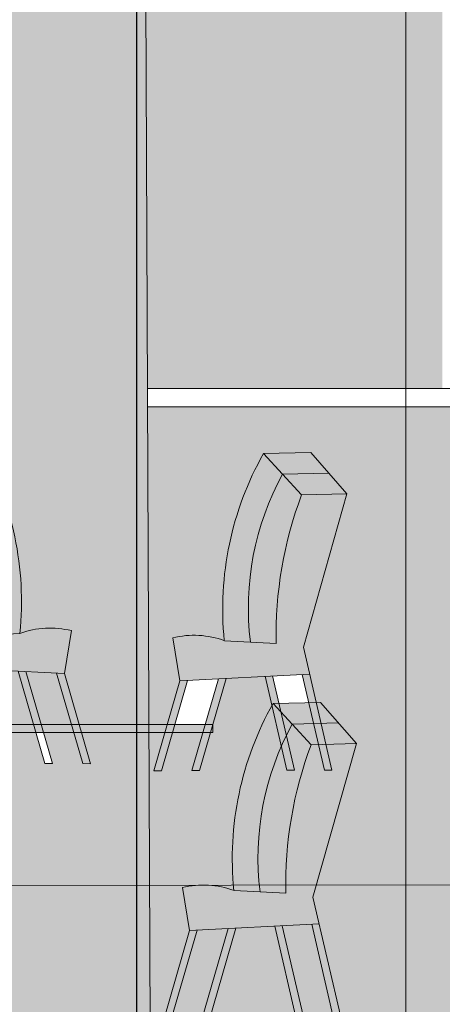
# Model space of a CAD drawing. Units: millimetres. Extents: x 11032 to 26788, y 3406 to 24505.
# Tile 10 of 78: x 16566 to 17145, y 7421 to 8770. Entities that reach past the tile are written whole.
import ezdxf

# ---------------------------------------------------------------- set-up
doc = ezdxf.new("R2010")
doc.units = ezdxf.units.MM
doc.header["$MEASUREMENT"] = 0
for name, color, linetype, lineweight in [('A-ANNO-DIMS', 2, 'Continuous', 18), ('A-FURN', 8, 'Continuous', 13), ('A-FURN-PATT', 8, 'Continuous', 13), ('A-GLAZ', 250, 'Continuous', 20), ('A-WALL-INTR', 8, 'Continuous', 18)]:
    doc.layers.add(name, color=color, linetype=linetype, lineweight=lineweight)
doc.layers.add('A-GLAZ-FRAM-PATT', color=250, linetype='Continuous', lineweight=13, true_color=0x262627)
doc.layers.add('A-WALL-INTR-PATT', color=251, linetype='Continuous', lineweight=13, true_color=0x6c6b6a)
doc.styles.get("Standard").update_dxf_attribs({"font": 'arial.ttf'})
doc.dimstyles.get("Standard").update_dxf_attribs({"dimtxt": 150, "dimasz": 100, "dimexe": 10, "dimexo": 5, "dimgap": 5, "dimtad": 0, "dimtih": 1, "dimtoh": 1, "dimdec": 0, "dimzin": 0, "dimdsep": 46, "dimtxsty": 'Standard', "dimcen": 0.09, "dimadec": 0, "dimazin": 0, "dimtfac": 1, "dimtdec": 0, "dimtofl": 0, "dimtmove": 0, "dimatfit": 3, "dimfxl": 1, "dimtolj": 1, "dimtzin": 0, "dimarcsym": 0})

# ---------------------------------------------------------------- blocks, each defined once
blk = doc.blocks.new('DINING-CHAIR-ELEV')
blk.add_line((228.7, 123.4), (51, 132.6))
for points in [[(0, 379.5), (49.4, 435.9), (114.1, 434.5)], [(61.2, 132.1), (30.8, 1.2), (20.5, 1.2), (59.5, 169.3), (0, 379.5), (61.9, 377.9)], [(111.9, 129.5), (82.1, 0.9), (71.8, 1), (101.8, 130)], [(165.3, 126.7), (201.8, 0.3), (212.2, 0.3), (175.8, 126.2)]]:
    blk.add_lwpolyline(points)
for points in [[(218.1, 124), (253.9, 0.1), (264.3, 0), (228.7, 123.4), (238.3, 182.2, 0.148451), (167.5, 178.3), (96.6, 174.5, 0.097012), (61.9, 377.9), (114.1, 434.5, -0.154833), (167.8, 178.5)], [(132, 176.4, 0.156877), (88, 406.2), (24.7, 407.7)]]:
    blk.add_lwpolyline(points, format="xyb")
blk = doc.blocks.new('DINING-TABLE-ELEV')
blk.add_lwpolyline([(0, 0), (986.1, 0), (986.1, 11.1), (0, 11.1)], close=True)
blk = doc.blocks.new('*D17')
at = {"layer": 'A-ANNO-DIMS', "color": 0, "lineweight": -2, "transparency": 16777216}
for p, q in [((15472.4, 7380.1), (15472.4, 7309.7)), ((15736.7, 7380.1), (15736.7, 7309.7)), ((15572.4, 7319.7), (15636.7, 7319.7)), ((15736.7, 7319.7), (15836.7, 7319.7))]:
    blk.add_line(p, q, dxfattribs=at)
at = {"layer": 'A-ANNO-DIMS', "color": 0, "transparency": 16777216}
for points in [[(15572.4, 7336.4), (15572.4, 7303), (15472.4, 7319.7)], [(15636.7, 7336.4), (15636.7, 7303), (15736.7, 7319.7)]]:
    blk.add_solid(points, dxfattribs=at)
at = {"layer": 'Defpoints', "color": 0, "transparency": 16777216}
for p in [(15472.4, 7385.1), (15736.7, 7385.1), (15736.7, 7319.7)]:
    blk.add_point(p, dxfattribs=at)
at = {"layer": 'A-ANNO-DIMS', "color": 0, "transparency": 16777216, "insert": (16266.4, 7319.7), "char_height": 150, "attachment_point": 5}
blk.add_mtext('\\A1;264 TYP.', dxfattribs=at)
blk = doc.blocks.new('*D36')
at = {"layer": 'A-ANNO-DIMS', "color": 0, "lineweight": -2, "transparency": 16777216}
for p, q in [((12301.3, 17115.9), (12301.3, 24416.9)), ((12401.3, 24406.9), (18569.2, 24406.9)), ((25297.4, 24406.9), (19129.5, 24406.9)), ((25397.4, 4466.4), (25397.4, 24416.9))]:
    blk.add_line(p, q, dxfattribs=at)
at = {"layer": 'A-ANNO-DIMS', "color": 0, "transparency": 16777216}
for points in [[(12401.3, 24423.5), (12401.3, 24390.2), (12301.3, 24406.9)], [(25297.4, 24423.5), (25297.4, 24390.2), (25397.4, 24406.9)]]:
    blk.add_solid(points, dxfattribs=at)
at = {"layer": 'Defpoints', "color": 0, "transparency": 16777216}
for p in [(25397.4, 24406.9), (12301.3, 17110.9), (25397.4, 4461.4)]:
    blk.add_point(p, dxfattribs=at)
at = {"layer": 'A-ANNO-DIMS', "color": 0, "transparency": 16777216, "insert": (18849.3, 24406.9), "char_height": 150, "attachment_point": 5}
blk.add_mtext('\\A1;13096', dxfattribs=at)
blk = doc.blocks.new('*D37')
at = {"layer": 'A-ANNO-DIMS', "color": 0, "lineweight": -2, "transparency": 16777216}
for p, q in [((18087.7, 23450.4), (11334.8, 23450.4)), ((11344.8, 23350.4), (11344.8, 14037.5)), ((11344.8, 4561.4), (11344.8, 13874.3)), ((12927.7, 4461.4), (11334.8, 4461.4))]:
    blk.add_line(p, q, dxfattribs=at)
at = {"layer": 'A-ANNO-DIMS', "color": 0, "transparency": 16777216}
for points in [[(11328.1, 23350.4), (11361.4, 23350.4), (11344.8, 23450.4)], [(11328.1, 4561.4), (11361.4, 4561.4), (11344.8, 4461.4)]]:
    blk.add_solid(points, dxfattribs=at)
at = {"layer": 'Defpoints', "color": 0, "transparency": 16777216}
for p in [(11344.8, 23450.4), (18092.7, 23450.4), (12932.7, 4461.4)]:
    blk.add_point(p, dxfattribs=at)
at = {"layer": 'A-ANNO-DIMS', "color": 0, "transparency": 16777216, "insert": (11344.8, 13955.9), "char_height": 150, "attachment_point": 5}
blk.add_mtext('\\A1;18989', dxfattribs=at)
blk = doc.blocks.new('*D49')
at = {"layer": 'A-ANNO-DIMS', "color": 0, "lineweight": -2, "transparency": 16777216}
for p, q in [((17953.5, 10206.4), (17953.5, 3494.9)), ((14996.4, 6406.4), (14996.4, 3494.9)), ((15096.4, 3504.9), (16244.7, 3504.9)), ((17853.5, 3504.9), (16705.2, 3504.9))]:
    blk.add_line(p, q, dxfattribs=at)
at = {"layer": 'A-ANNO-DIMS', "color": 0, "transparency": 16777216}
for points in [[(15096.4, 3521.6), (15096.4, 3488.2), (14996.4, 3504.9)], [(17853.5, 3521.6), (17853.5, 3488.2), (17953.5, 3504.9)]]:
    blk.add_solid(points, dxfattribs=at)
at = {"layer": 'Defpoints', "color": 0, "transparency": 16777216}
for p in [(17953.5, 10211.4), (14996.4, 6411.4), (17953.5, 3504.9)]:
    blk.add_point(p, dxfattribs=at)
at = {"layer": 'A-ANNO-DIMS', "color": 0, "transparency": 16777216, "insert": (16474.9, 3504.9), "char_height": 150, "attachment_point": 5}
blk.add_mtext('\\A1;2957', dxfattribs=at)
blk = doc.blocks.new('*D57')
at = {"layer": 'A-ANNO-DIMS', "color": 0, "lineweight": -2, "transparency": 16777216}
for p, q in [((14994.7, 7266.4), (14994.7, 24416.9)), ((15094.7, 24406.9), (17716, 24406.9)), ((20794.7, 24406.9), (18173.4, 24406.9)), ((20894.7, 7266.4), (20894.7, 24416.9))]:
    blk.add_line(p, q, dxfattribs=at)
at = {"layer": 'A-ANNO-DIMS', "color": 0, "transparency": 16777216}
for points in [[(15094.7, 24423.5), (15094.7, 24390.2), (14994.7, 24406.9)], [(20794.7, 24423.5), (20794.7, 24390.2), (20894.7, 24406.9)]]:
    blk.add_solid(points, dxfattribs=at)
at = {"layer": 'Defpoints', "color": 0, "transparency": 16777216}
for p in [(20894.7, 24406.9), (14994.7, 7261.4), (20894.7, 7261.4)]:
    blk.add_point(p, dxfattribs=at)
at = {"layer": 'A-ANNO-DIMS', "color": 0, "transparency": 16777216, "insert": (17944.7, 24406.9), "char_height": 150, "attachment_point": 5}
blk.add_mtext('\\A1;5900', dxfattribs=at)
blk = doc.blocks.new('*D66')
at = {"layer": 'A-ANNO-DIMS', "color": 0, "lineweight": -2, "transparency": 16777216}
for p, q in [((16725.9, 10296), (16725.9, 3494.9)), ((19150.9, 10296), (19150.9, 3494.9)), ((16825.9, 3504.9), (17707.6, 3504.9)), ((19050.9, 3504.9), (18169.3, 3504.9))]:
    blk.add_line(p, q, dxfattribs=at)
at = {"layer": 'A-ANNO-DIMS', "color": 0, "transparency": 16777216}
for points in [[(16825.9, 3521.6), (16825.9, 3488.2), (16725.9, 3504.9)], [(19050.9, 3521.6), (19050.9, 3488.2), (19150.9, 3504.9)]]:
    blk.add_solid(points, dxfattribs=at)
at = {"layer": 'Defpoints', "color": 0, "transparency": 16777216}
for p in [(16725.9, 10301), (19150.9, 10301), (19150.9, 3504.9)]:
    blk.add_point(p, dxfattribs=at)
at = {"layer": 'A-ANNO-DIMS', "color": 0, "transparency": 16777216, "insert": (17938.4, 3504.9), "char_height": 150, "attachment_point": 5}
blk.add_mtext('\\A1;2425', dxfattribs=at)
blk = doc.blocks.new('*D69')
at = {"layer": 'A-ANNO-DIMS', "color": 0, "lineweight": -2, "transparency": 16777216}
for p, q in [((13957, 9938), (14057, 9938)), ((14057, 9938), (15432.5, 8991)), ((17944.6, 7261.4), (17944.8, 7261.4)), ((17944.7, 7261.3), (17944.7, 7261.5))]:
    blk.add_line(p, q, dxfattribs=at)
at = {"layer": 'A-ANNO-DIMS', "color": 0, "transparency": 16777216}
blk.add_solid([(15442, 9004.7), (15423.1, 8977.2), (15514.9, 8934.2)], dxfattribs=at)
at = {"layer": 'Defpoints', "color": 0, "transparency": 16777216}
for p in [(15514.9, 8934.2), (17944.7, 7261.4)]:
    blk.add_point(p, dxfattribs=at)
at = {"layer": 'A-ANNO-DIMS', "color": 0, "transparency": 16777216, "insert": (13494, 9938), "char_height": 150, "attachment_point": 5}
blk.add_mtext('\\A1;2X R2950', dxfattribs=at)

msp = doc.modelspace()

# ---------------------------------------------------------------- hatches: boundary and pattern name
at = {"layer": 'A-FURN-PATT'}
h = msp.add_hatch(color=256, dxfattribs=at)
h.set_gradient(color1=(82, 15, 16), color2=(153, 0, 38), name='CURVED')
h.paths.add_polyline_path([(16952.125, 8119), (16926.017, 8147.32, 0.15687748), (16881.989, 7917.509), (16917.415, 7915.583, -0.09701208)], flags=0)
h.paths.add_polyline_path([(16899.908, 8175.64), (16964.58, 8177.046), (17014.03, 8120.657), (16954.484, 7910.365), (16972.017, 7834.84), (16977.75, 7834.965), (17027.199, 7778.576), (16967.653, 7568.284), (17006.665, 7400.238), (16996.411, 7400.187), (16966.016, 7531.114), (16925.439, 7529.018), (16955.395, 7399.983), (16945.141, 7399.932), (16915.295, 7528.494), (16861.916, 7525.736), (16825.435, 7399.337), (16815.012, 7399.285), (16851.35, 7525.19), (16809.087, 7523.007), (16773.319, 7399.078), (16762.896, 7399.026), (16798.521, 7522.461), (16788.882, 7581.207, -0.14766935), (16859.382, 7577.482, -0.15281323), (16911.41, 7830.579), (16902.125, 7870.575), (16848.746, 7867.817), (16830.506, 7804.617), (16830.506, 7793.515), (16827.302, 7793.515), (16812.265, 7741.418), (16801.842, 7741.366), (16816.893, 7793.515), (16775.261, 7793.515), (16760.15, 7741.159), (16749.727, 7741.107), (16764.853, 7793.515), (16650.704, 7793.515), (16662.994, 7750.932), (16652.571, 7750.983), (16640.296, 7793.515), (16598.663, 7793.515), (16610.879, 7751.191), (16600.455, 7751.242), (16588.255, 7793.515), (16490.425, 7793.515), (16480.749, 7751.837), (16470.495, 7751.888), (16480.159, 7793.515), (16443.833, 7793.515, -0.10940509), (16465.746, 7607.731, -0.14766935), (16536.246, 7611.456), (16526.606, 7552.71), (16562.232, 7429.275), (16551.809, 7429.327), (16516.041, 7553.255), (16473.778, 7555.439), (16510.116, 7429.534), (16499.693, 7429.586), (16463.212, 7555.985), (16409.833, 7558.743), (16379.987, 7430.181), (16369.733, 7430.232), (16394.704, 7537.793), (16394.704, 7559.524), (16359.112, 7561.363), (16328.717, 7430.435), (16318.463, 7430.486), (16344.704, 7543.521), (16344.704, 7643.635), (16302.264, 7793.515), (16205.738, 7793.515), (16227.021, 7719.773), (16216.598, 7719.825), (16195.329, 7793.515), (16153.697, 7793.515), (16174.905, 7720.032), (16164.482, 7720.084), (16143.289, 7793.515), (15844.423, 7793.515), (15844.423, 7804.617), (16140.084, 7804.617), (16128.001, 7846.483), (16191.395, 7843.208), (16201.035, 7901.954, 0.14845082), (16130.184, 7898.102), (16059.333, 7894.25, 0.09701208), (16024.622, 8097.666), (16076.839, 8154.307, -0.15483335), (16130.535, 7898.229, -0.14766935), (16201.035, 7901.954), (16191.395, 7843.208), (16202.533, 7804.617), (16299.12, 7804.617), (16297.929, 7808.825), (16347.378, 7865.214), (16412.05, 7863.808, -0.02954963), (16434.494, 7817.915), (16458.237, 7920.19), (16398.691, 8130.481), (16448.141, 8186.871), (16512.813, 8185.465, -0.15483335), (16566.508, 7929.387, -0.14766935), (16637.008, 7933.112), (16627.369, 7874.366), (16647.499, 7804.617), (16742.939, 7804.617), (16741.107, 8264.696), (17994.704, 8264.696), (17994.704, 7796.661), (18112.02, 7796.661), (18134.447, 7874.366), (18124.807, 7933.112, -0.14766935), (18195.307, 7929.387, -0.15483335), (18249.003, 8185.465), (18313.675, 8186.871), (18363.124, 8130.481), (18303.578, 7920.19), (18311.087, 7887.847, -0.02730168), (18332.016, 7930.161), (18396.688, 7931.567), (18446.137, 7875.177), (18423.905, 7796.661), (18470.25, 7796.661), (18470.25, 7785.559), (18420.761, 7785.559), (18386.591, 7664.886), (18425.604, 7496.839), (18415.35, 7496.788), (18384.955, 7627.716), (18344.377, 7625.62), (18374.333, 7496.584), (18364.079, 7496.533), (18334.233, 7625.095), (18280.854, 7622.338), (18244.373, 7495.938), (18233.95, 7495.887), (18270.288, 7621.792), (18228.026, 7619.608), (18192.257, 7495.679), (18181.834, 7495.628), (18217.46, 7619.062), (18207.82, 7677.808, -0.14766935), (18278.32, 7674.083, -0.05141811), (18278.516, 7762.821), (18273.237, 7785.559), (18171.265, 7785.559), (18161.36, 7751.242), (18150.937, 7751.191), (18160.856, 7785.559), (18119.224, 7785.559), (18109.244, 7750.983), (18098.821, 7750.932), (18108.815, 7785.559), (17852.794, 7785.559), (17866.18, 7739.181), (17855.756, 7739.233), (17842.386, 7785.559), (17800.753, 7785.559), (17814.064, 7739.44), (17803.641, 7739.492), (17790.345, 7785.559), (17694.491, 7785.559), (17685.986, 7748.922, -0.08827454), (17728.687, 7746.171), (17719.047, 7687.425), (17754.673, 7563.99), (17744.25, 7564.042), (17708.482, 7687.971), (17666.219, 7690.154), (17702.557, 7564.249), (17692.134, 7564.301), (17655.653, 7690.7), (17602.274, 7693.458), (17572.428, 7564.896), (17562.174, 7564.947), (17592.13, 7693.982), (17551.553, 7696.078), (17521.158, 7565.151), (17510.903, 7565.202), (17549.916, 7733.248), (17535.103, 7785.559), (17484.167, 7785.559), (17484.167, 7796.661), (17531.96, 7796.661), (17490.37, 7943.54), (17539.819, 7999.929), (17604.491, 7998.523, -0.08024859), (17652.289, 7869.096), (17661.422, 7908.439), (17601.876, 8118.731), (17651.326, 8175.12), (17715.998, 8173.714, -0.15483335), (17769.694, 7917.637, -0.14766935), (17840.194, 7921.361), (17830.554, 7862.615), (17849.59, 7796.661), (17894.704, 7796.661), (17894.704, 8239.696), (16741.207, 8239.696), (16742.939, 7804.617), (16768.057, 7804.617), (16785.352, 7864.542), (16775.713, 7923.288, -0.14766935), (16846.212, 7919.563, -0.15483335)], flags=17)
h.paths.add_polyline_path([(16899.908, 8175.64), (16964.58, 8177.046), (17014.03, 8120.657), (16954.484, 7910.365), (16993.496, 7742.318), (16983.242, 7742.267), (16952.847, 7873.195), (16912.27, 7871.099), (16942.225, 7742.064), (16931.971, 7742.013), (16902.125, 7870.575), (16848.746, 7867.817), (16812.265, 7741.418), (16801.842, 7741.366), (16838.181, 7867.271), (16795.918, 7865.087), (16760.15, 7741.159), (16749.727, 7741.107), (16785.352, 7864.542), (16775.713, 7923.288, -0.14766935), (16846.212, 7919.563, -0.15483335)], flags=0)
h.paths.add_polyline_path([(16899.908, 8175.64), (16964.58, 8177.046), (17014.03, 8120.657), (16954.484, 7910.365), (16972.017, 7834.84), (16977.75, 7834.965), (17027.199, 7778.576), (16967.653, 7568.284), (17006.665, 7400.238), (16996.411, 7400.187), (16966.016, 7531.114), (16925.439, 7529.018), (16955.395, 7399.983), (16945.141, 7399.932), (16915.295, 7528.494), (16861.916, 7525.736), (16825.435, 7399.337), (16815.012, 7399.285), (16851.35, 7525.19), (16809.087, 7523.007), (16773.319, 7399.078), (16762.896, 7399.026), (16798.521, 7522.461), (16788.882, 7581.207, -0.14766935), (16859.382, 7577.482, -0.15281323), (16911.41, 7830.579), (16902.125, 7870.575), (16848.746, 7867.817), (16830.506, 7804.617), (16830.506, 7793.515), (16827.302, 7793.515), (16812.265, 7741.418), (16801.842, 7741.366), (16816.893, 7793.515), (16775.261, 7793.515), (16760.15, 7741.159), (16749.727, 7741.107), (16764.853, 7793.515), (16650.704, 7793.515), (16662.994, 7750.932), (16652.571, 7750.983), (16640.296, 7793.515), (16598.663, 7793.515), (16610.879, 7751.191), (16600.455, 7751.242), (16588.255, 7793.515), (16490.425, 7793.515), (16480.749, 7751.837), (16470.495, 7751.888), (16480.159, 7793.515), (16443.833, 7793.515, -0.10940509), (16465.746, 7607.731, -0.14766935), (16536.246, 7611.456), (16526.606, 7552.71), (16562.232, 7429.275), (16551.809, 7429.327), (16516.041, 7553.255), (16473.778, 7555.439), (16510.116, 7429.534), (16499.693, 7429.586), (16463.212, 7555.985), (16409.833, 7558.743), (16379.987, 7430.181), (16369.733, 7430.232), (16394.704, 7537.793), (16394.704, 7559.524), (16359.112, 7561.363), (16328.717, 7430.435), (16318.463, 7430.486), (16344.704, 7543.521), (16344.704, 7643.635), (16302.264, 7793.515), (16205.738, 7793.515), (16227.021, 7719.773), (16216.598, 7719.825), (16195.329, 7793.515), (16153.697, 7793.515), (16174.905, 7720.032), (16164.482, 7720.084), (16143.289, 7793.515), (15844.423, 7793.515), (15844.423, 7804.617), (16140.084, 7804.617), (16128.001, 7846.483), (16191.395, 7843.208), (16201.035, 7901.954, 0.14845082), (16130.184, 7898.102), (16059.333, 7894.25, 0.09701208), (16024.622, 8097.666), (16076.839, 8154.307, -0.15483335), (16130.535, 7898.229, -0.14766935), (16201.035, 7901.954), (16191.395, 7843.208), (16202.533, 7804.617), (16299.12, 7804.617), (16297.929, 7808.825), (16347.378, 7865.214), (16412.05, 7863.808, -0.02954963), (16434.494, 7817.915), (16458.237, 7920.19), (16398.691, 8130.481), (16448.141, 8186.871), (16512.813, 8185.465, -0.15483335), (16566.508, 7929.387, -0.14766935), (16637.008, 7933.112), (16627.369, 7874.366), (16647.499, 7804.617), (16742.939, 7804.617), (16741.207, 8239.696), (16741.107, 8264.696), (17994.704, 8264.696), (17994.704, 7796.661), (18112.02, 7796.661), (18134.447, 7874.366), (18124.807, 7933.112, -0.14766935), (18195.307, 7929.387, -0.15483335), (18249.003, 8185.465), (18313.675, 8186.871), (18363.124, 8130.481), (18303.578, 7920.19), (18311.087, 7887.847, -0.02730168), (18332.016, 7930.161), (18396.688, 7931.567), (18446.137, 7875.177), (18423.905, 7796.661), (18470.25, 7796.661), (18470.25, 7785.559), (18420.761, 7785.559), (18386.591, 7664.886), (18425.604, 7496.839), (18415.35, 7496.788), (18384.955, 7627.716), (18344.377, 7625.62), (18374.333, 7496.584), (18364.079, 7496.533), (18334.233, 7625.095), (18280.854, 7622.338), (18244.373, 7495.938), (18233.95, 7495.887), (18270.288, 7621.792), (18228.026, 7619.608), (18192.257, 7495.679), (18181.834, 7495.628), (18217.46, 7619.062), (18207.82, 7677.808, -0.14766935), (18278.32, 7674.083, -0.05141811), (18278.516, 7762.821), (18273.237, 7785.559), (18171.265, 7785.559), (18161.36, 7751.242), (18150.937, 7751.191), (18160.856, 7785.559), (18119.224, 7785.559), (18109.244, 7750.983), (18098.821, 7750.932), (18108.815, 7785.559), (17852.794, 7785.559), (17866.18, 7739.181), (17855.756, 7739.233), (17842.386, 7785.559), (17800.753, 7785.559), (17814.064, 7739.44), (17803.641, 7739.492), (17790.345, 7785.559), (17694.491, 7785.559), (17685.986, 7748.922, -0.08827454), (17728.687, 7746.171), (17719.047, 7687.425), (17754.673, 7563.99), (17744.25, 7564.042), (17708.482, 7687.971), (17666.219, 7690.154), (17702.557, 7564.249), (17692.134, 7564.301), (17655.653, 7690.7), (17602.274, 7693.458), (17572.428, 7564.896), (17562.174, 7564.947), (17592.13, 7693.982), (17551.553, 7696.078), (17521.158, 7565.151), (17510.903, 7565.202), (17549.916, 7733.248), (17535.103, 7785.559), (17484.167, 7785.559), (17484.167, 7796.661), (17531.96, 7796.661), (17490.37, 7943.54), (17539.819, 7999.929), (17604.491, 7998.523, -0.08024859), (17652.289, 7869.096), (17661.422, 7908.439), (17601.876, 8118.731), (17651.326, 8175.12), (17715.998, 8173.714, -0.15483335), (17769.694, 7917.637, -0.14766935), (17840.194, 7921.361), (17830.554, 7862.615), (17849.59, 7796.661), (17894.704, 7796.661), (17894.704, 8239.696), (16741.207, 8239.696), (16742.939, 7804.617), (16768.057, 7804.617), (16785.352, 7864.542), (16775.713, 7923.288, -0.14766935), (16846.212, 7919.563, -0.15483335)], flags=17)
h = msp.add_hatch(color=256, dxfattribs=at)
h.set_gradient(color1=(153, 27, 30), color2=(153, 38, 0), name='SPHERICAL')
h.paths.add_polyline_path([(15534.344, 7763), (15472.44, 7764.657), (15531.986, 7554.365), (15523.479, 7517.719), (15640.736, 7511.661), (15653.713, 7567.556, 0.02952029), (15639.906, 7563.436), (15569.055, 7559.583, 0.09701208)], flags=16)
h.paths.add_polyline_path([(15560.453, 7791.32), (15534.344, 7763, -0.09701208), (15569.055, 7559.583), (15604.48, 7561.509, 0.15687748)], flags=16)
h.paths.add_polyline_path([(15586.562, 7819.64), (15560.453, 7791.32, -0.15687748), (15604.48, 7561.509), (15640.246, 7563.454, 0.15489802)], flags=17)
h.paths.add_polyline_path([(15560.453, 7791.32), (15497.165, 7792.851), (15472.44, 7764.657), (15534.344, 7763)], flags=16)
h.paths.add_polyline_path([(15586.562, 7819.64), (15521.889, 7821.046), (15497.165, 7792.851), (15560.453, 7791.32)], flags=17)
h.paths.add_polyline_path([(15790.874, 7662.689, 0.02146895), (15780.879, 7659.53), (15710.028, 7655.677, 0.09701208), (15675.317, 7859.094), (15665.772, 7859.35), (15665.799, 7675.745), (15672.959, 7650.459), (15665.807, 7619.654), (15665.808, 7613.744), (15790.755, 7607.288)], flags=17)
h.paths.add_polyline_path([(15665.772, 7859.35), (15613.413, 7860.751), (15665.799, 7675.745)], flags=16)
h.paths.add_polyline_path([(15701.426, 7887.414), (15665.767, 7888.277), (15665.772, 7859.35), (15675.317, 7859.094)], flags=16)
h.paths.add_polyline_path([(15727.534, 7915.735), (15665.763, 7917.077), (15665.767, 7888.277), (15701.426, 7887.414)], flags=17)
h.paths.add_polyline_path([(15665.763, 7917.077), (15662.862, 7917.14), (15638.137, 7888.946), (15665.767, 7888.277)], flags=17)
h.paths.add_polyline_path([(15665.767, 7888.277), (15638.137, 7888.946), (15613.413, 7860.751), (15665.772, 7859.35)], flags=16)
h.paths.add_polyline_path([(15701.426, 7887.414), (15675.317, 7859.094, -0.09701208), (15710.028, 7655.677), (15745.453, 7657.604, 0.15687748)], flags=16)
h.paths.add_polyline_path([(15844.495, 7664.925), (15844.384, 7864.461), (15821.312, 7945.94), (15870.762, 8002.329), (15935.434, 8000.923, -0.11959168), (15991.005, 7804.617), (16002.667, 7804.617), (16022.264, 7889.032), (15962.718, 8099.323), (16024.622, 8097.666), (16076.839, 8154.307, -0.15483335), (16130.535, 7898.229, -0.14766935), (16201.035, 7901.954), (16191.395, 7843.208), (16202.533, 7804.617), (16299.12, 7804.617), (16297.929, 7808.825), (16347.378, 7865.214), (16412.05, 7863.808, -0.02954963), (16434.494, 7817.915), (16458.237, 7920.19), (16398.691, 8130.481), (16460.595, 8128.825), (16512.813, 8185.465, -0.15483335), (16566.508, 7929.387, -0.14766935), (16637.008, 7933.112), (16627.369, 7874.366), (16647.499, 7804.617), (16830.506, 7804.617), (16830.506, 7793.515), (16650.704, 7793.515), (16662.994, 7750.932), (16652.571, 7750.983), (16640.296, 7793.515), (16490.425, 7793.515), (16480.749, 7751.837), (16470.495, 7751.888), (16480.159, 7793.515), (16443.833, 7793.515, -0.10940509), (16465.746, 7607.731, -0.14766935), (16536.246, 7611.456), (16526.606, 7552.71), (16562.232, 7429.275), (16551.809, 7429.327), (16516.041, 7553.255), (16473.778, 7555.439), (16510.116, 7429.534), (16499.693, 7429.586), (16463.212, 7555.985), (16409.833, 7558.743), (16379.987, 7430.181), (16369.733, 7430.232), (16394.704, 7537.793), (16394.704, 7559.524), (16359.112, 7561.363), (16328.717, 7430.435), (16318.463, 7430.486), (16344.704, 7543.521), (16344.704, 7643.635), (16302.264, 7793.515), (16205.738, 7793.515), (16227.021, 7719.773), (16216.598, 7719.825), (16195.329, 7793.515), (16153.697, 7793.515), (16174.905, 7720.032), (16164.482, 7720.084), (16143.289, 7793.515), (16061.685, 7793.515), (16051.641, 7750.248, -0.01671442), (16059.629, 7748.571), (16049.99, 7689.825), (16085.615, 7566.39), (16075.192, 7566.442), (16039.424, 7690.371), (15997.161, 7692.554), (16033.5, 7566.649), (16023.077, 7566.701), (15986.595, 7693.1), (15933.216, 7695.858), (15903.371, 7567.296), (15893.116, 7567.347), (15923.072, 7696.382), (15882.495, 7698.478), (15852.409, 7568.882), (15877.716, 7481.201), (15867.293, 7481.253), (15842.372, 7567.599), (15841.846, 7567.602), (15842.08, 7568.609), (15831.524, 7605.182), (15790.755, 7607.288), (15790.744, 7602.228), (15825.6, 7481.46), (15815.177, 7481.512), (15778.696, 7607.911), (15725.317, 7610.669), (15701.389, 7507.6), (15736.743, 7385.107), (15726.32, 7385.159), (15696.749, 7487.614), (15695.471, 7482.107), (15685.217, 7482.158), (15691.06, 7507.327), (15690.552, 7509.088), (15650.881, 7511.137), (15649.743, 7506.234), (15684.627, 7385.366), (15674.204, 7385.418), (15645.103, 7486.248), (15644.2, 7482.362), (15633.946, 7482.413), (15639.413, 7505.961), (15637.723, 7511.817), (15584.344, 7514.575), (15554.498, 7386.013), (15544.244, 7386.064), (15574.2, 7515.099), (15533.623, 7517.195), (15503.228, 7386.268), (15492.974, 7386.319), (15531.986, 7554.365), (15472.44, 7764.657), (15497.165, 7792.851), (15521.889, 7821.046), (15586.562, 7819.64, -0.15483335), (15640.257, 7563.563, -0.02875494), (15653.713, 7567.556), (15665.807, 7619.654), (15665.799, 7675.745), (15613.413, 7860.751), (15638.137, 7888.946), (15662.862, 7917.14), (15665.763, 7917.077), (15727.534, 7915.735, -0.15483335), (15781.23, 7659.657, -0.13222632)])
h = msp.add_hatch(color=256, dxfattribs=at)
h.set_gradient(color1=(153, 27, 30), color2=(153, 38, 0), name='SPHERICAL')
h.paths.add_polyline_path([(15710.028, 7655.677), (15745.453, 7657.604, 0.15687748), (15701.426, 7887.414), (15675.317, 7859.094, -0.09701208)], flags=16)
h.paths.add_polyline_path([(15790.755, 7607.288), (15790.874, 7662.689, 0.02146895), (15780.879, 7659.53), (15710.028, 7655.677, 0.09701208), (15675.317, 7859.094), (15665.772, 7859.35), (15665.799, 7675.745), (15672.959, 7650.459), (15665.807, 7619.654), (15665.808, 7613.744)], flags=17)
h.paths.add_polyline_path([(15653.713, 7567.556), (15665.807, 7619.654), (15665.799, 7675.745), (15613.413, 7860.751), (15662.862, 7917.14), (15727.534, 7915.735, -0.15483335), (15781.23, 7659.657, -0.13222632), (15844.495, 7664.925), (15844.384, 7864.461), (15821.312, 7945.94), (15883.216, 7944.283), (15935.434, 8000.923, -0.11959168), (15991.005, 7804.617), (16002.667, 7804.617), (16022.264, 7889.032), (15962.718, 8099.323), (16024.622, 8097.666), (16076.839, 8154.307, -0.15483335), (16130.535, 7898.229, -0.14766935), (16201.035, 7901.954), (16191.395, 7843.208), (16202.533, 7804.617), (16830.506, 7804.617), (16830.506, 7793.515), (16205.738, 7793.515), (16227.021, 7719.773), (16216.598, 7719.825), (16195.329, 7793.515), (16153.697, 7793.515), (16174.905, 7720.032), (16164.482, 7720.084), (16143.289, 7793.515), (16061.685, 7793.515), (16051.641, 7750.248, -0.01671442), (16059.629, 7748.571), (16049.99, 7689.825), (16085.615, 7566.39), (16075.192, 7566.442), (16039.424, 7690.371), (15997.161, 7692.554), (16033.5, 7566.649), (16023.077, 7566.701), (15986.595, 7693.1), (15933.216, 7695.858), (15903.371, 7567.296), (15893.116, 7567.347), (15923.072, 7696.382), (15882.495, 7698.478), (15852.409, 7568.882), (15877.716, 7481.201), (15867.293, 7481.253), (15842.372, 7567.599), (15841.846, 7567.602), (15842.08, 7568.609), (15831.524, 7605.182), (15790.755, 7607.288), (15790.744, 7602.228), (15825.6, 7481.46), (15815.177, 7481.512), (15778.696, 7607.911), (15725.317, 7610.669), (15701.389, 7507.6), (15736.743, 7385.107), (15726.32, 7385.159), (15696.749, 7487.614), (15695.471, 7482.107), (15685.217, 7482.158), (15705.262, 7568.502, 0.08416849), (15664.448, 7569.579), (15644.2, 7482.362), (15633.946, 7482.413), (15653.713, 7567.556, 0.02952029), (15639.906, 7563.436), (15569.055, 7559.583, 0.09701208), (15534.344, 7763), (15472.44, 7764.657), (15521.889, 7821.046), (15586.562, 7819.64, -0.15483335), (15640.257, 7563.563, -0.02875494)])
h = msp.add_hatch(color=256, dxfattribs=at)
h.set_gradient(color1=(82, 15, 16), color2=(153, 0, 38), name='CURVED')
h.paths.add_polyline_path([(16913.077, 7833.559), (16977.75, 7834.965), (17027.199, 7778.576), (16967.653, 7568.284), (17006.665, 7400.238), (16996.411, 7400.187), (16966.016, 7531.114), (16925.439, 7529.018), (16955.395, 7399.983), (16945.141, 7399.932), (16915.295, 7528.494), (16861.916, 7525.736), (16825.435, 7399.337), (16815.012, 7399.285), (16851.35, 7525.19), (16809.087, 7523.007), (16773.319, 7399.078), (16762.896, 7399.026), (16798.521, 7522.461), (16788.882, 7581.207, -0.14766935), (16859.382, 7577.482, -0.15483335)])
h.paths.add_polyline_path([(16881.989, 7917.509), (16917.415, 7915.583, -0.09701208), (16952.125, 8119), (16926.017, 8147.32, 0.15687748)])
at = {"layer": 'A-GLAZ-FRAM-PATT'}
h = msp.add_hatch(color=256, dxfattribs=at)
h.paths.add_polyline_path([(17944.704, 7311.399), (16344.704, 7311.399), (16344.704, 7261.399), (17944.704, 7261.399)], flags=17)
h.paths.add_polyline_path([(16344.704, 7311.399), (15045.135, 7311.399, -0.98290472), (20844.273, 7311.399), (19544.704, 7311.399), (19544.704, 7261.399), (20894.704, 7261.399, 0.51484406), (16985.951, 10051.255, 0.32026791), (14994.704, 7261.399), (16344.704, 7261.399)])
h.paths.add_polyline_path([(18744.704, 7311.399), (17944.704, 7311.399), (17944.704, 7261.399), (18744.704, 7261.399)], flags=17)
h.paths.add_polyline_path([(19544.704, 7311.399), (18744.704, 7311.399), (18744.704, 7261.399), (19544.704, 7261.399)], flags=17)
h.paths.add_polyline_path([(18694.704, 7361.399), (17994.704, 7361.399), (17994.704, 7311.399), (18694.704, 7311.399)], flags=17)
h.paths.add_polyline_path([(18744.704, 7361.399), (18694.704, 7361.399), (18694.704, 7311.399), (18744.704, 7311.399)], flags=17)
h.paths.add_polyline_path([(17194.704, 7361.399), (17144.704, 7361.399), (17144.704, 7311.399), (17194.704, 7311.399)], flags=17)
h.paths.add_polyline_path([(17431.432, 7361.399), (17194.704, 7361.399), (17194.704, 7311.399), (17431.699, 7311.399)], flags=17)
h.paths.add_polyline_path([(17894.704, 7361.399), (17431.432, 7361.399), (17431.699, 7311.399), (17894.704, 7311.399)], flags=17)
h.paths.add_polyline_path([(17944.704, 7361.399), (17894.704, 7361.399), (17894.704, 7311.399), (17944.704, 7311.399)], flags=17)
h.paths.add_polyline_path([(17994.704, 7361.399), (17944.704, 7361.399), (17944.704, 7311.399), (17994.704, 7311.399)], flags=17)
h = msp.add_hatch(color=256, dxfattribs=at)
h.paths.add_polyline_path([(16394.704, 9712.419, 0.00513365), (16344.704, 9680.076), (16344.704, 7862.164), (16347.378, 7865.214), (16394.704, 7864.185)])
h.paths.add_polyline_path([(17144.704, 10048.871, 0.02352245), (16886.403, 9961.399), (17094.704, 9961.399), (17094.704, 8264.696), (17144.704, 8264.696)])
h.paths.add_polyline_path([(18794.704, 9961.399), (19003.004, 9961.399, 0.02352245), (18744.704, 10048.871), (18744.704, 8264.696), (18794.704, 8264.696)])
h.paths.add_polyline_path([(19544.704, 9680.076, 0.00513365), (19494.704, 9712.419), (19494.704, 7793.43), (19544.704, 7793.43)])
h = msp.add_hatch(color=256, dxfattribs=at)
h.paths.add_polyline_path([(16734.609, 9896.863, 0.03337538), (16394.704, 9712.419), (16394.704, 7804.617), (16431.407, 7804.617), (16458.237, 7920.19), (16398.691, 8130.481), (16448.141, 8186.871), (16512.813, 8185.465, -0.15483335), (16566.508, 7929.387, -0.14766935), (16637.008, 7933.112), (16627.369, 7874.366), (16647.499, 7804.617), (16742.939, 7804.617)])
h.paths.add_polyline_path([(17094.704, 9961.399), (16886.403, 9961.399, 0.01422214), (16734.609, 9896.863), (16741.107, 8264.696), (17094.704, 8264.696)])
h.paths.add_polyline_path([(17417.202, 10027.292), (17194.704, 10011.399), (17194.704, 8264.696), (17426.61, 8264.696)])
h.paths.add_polyline_path([(17144.704, 8239.696), (17094.704, 8239.696), (17094.704, 7361.399), (16394.704, 7361.399), (16394.704, 7493.572), (16379.987, 7430.181), (16369.733, 7430.232), (16394.704, 7537.793), (16394.704, 7559.524), (16359.112, 7561.363), (16344.704, 7499.3), (16344.704, 7311.399), (17144.704, 7311.399)])
h.paths.add_polyline_path([(17194.704, 8239.696), (17144.704, 8239.696), (17144.704, 7361.399), (17194.704, 7361.399)])
at = {"layer": 'A-WALL-INTR-PATT'}
h = msp.add_hatch(color=256, dxfattribs=at)
h.paths.add_polyline_path([(15302.659, 8457.059, 0.02810018), (15185.248, 8153.253), (15233.282, 7717.599), (15314.374, 7311.399), (15467.334, 7311.399), (15381.661, 7740.545)])
h.paths.add_polyline_path([(16344.704, 7543.521), (16344.704, 7643.635), (16302.264, 7793.515), (16205.738, 7793.515), (16227.021, 7719.773), (16216.598, 7719.825), (16195.329, 7793.515), (16153.697, 7793.515), (16174.905, 7720.032), (16164.482, 7720.084), (16143.289, 7793.515), (16061.685, 7793.515), (16051.641, 7750.248, -0.01671442), (16059.629, 7748.571), (16049.99, 7689.825), (16085.615, 7566.39), (16075.192, 7566.442), (16039.424, 7690.371), (15997.161, 7692.554), (16033.5, 7566.649), (16023.077, 7566.701), (15986.595, 7693.1), (15933.216, 7695.858), (15903.371, 7567.296), (15893.116, 7567.347), (15923.072, 7696.382), (15882.495, 7698.478), (15852.409, 7568.882), (15877.716, 7481.201), (15867.293, 7481.253), (15844.553, 7560.041), (15844.691, 7311.399), (16344.704, 7311.399), (16344.704, 7499.3), (16328.717, 7430.435), (16318.463, 7430.486)])
h.paths.add_polyline_path([(16742.983, 7793.515), (16650.704, 7793.515), (16662.994, 7750.932), (16652.571, 7750.983), (16640.296, 7793.515), (16598.663, 7793.515), (16610.879, 7751.191), (16600.455, 7751.242), (16588.255, 7793.515), (16490.425, 7793.515), (16480.749, 7751.837), (16470.495, 7751.888), (16480.159, 7793.515), (16443.833, 7793.515, -0.10940509), (16465.746, 7607.731, -0.14766935), (16536.246, 7611.456), (16526.606, 7552.71), (16562.232, 7429.275), (16551.809, 7429.327), (16516.041, 7553.255), (16473.778, 7555.439), (16510.116, 7429.534), (16499.693, 7429.586), (16463.212, 7555.985), (16409.833, 7558.743), (16394.704, 7493.572), (16394.704, 7361.399), (16744.704, 7361.399)])
h.paths.add_polyline_path([(17094.704, 8239.696), (16741.207, 8239.696), (16742.939, 7804.617), (16768.057, 7804.617), (16785.352, 7864.542), (16775.713, 7923.288, -0.14766935), (16846.212, 7919.563, -0.15483335), (16899.908, 8175.64), (16964.58, 8177.046), (17014.03, 8120.657), (16954.484, 7910.365), (16972.017, 7834.84), (16977.75, 7834.965), (17027.199, 7778.576), (16967.653, 7568.284), (17006.665, 7400.238), (16996.411, 7400.187), (16966.016, 7531.114), (16925.439, 7529.018), (16955.395, 7399.983), (16945.141, 7399.932), (16915.295, 7528.494), (16861.916, 7525.736), (16825.435, 7399.337), (16815.012, 7399.285), (16851.35, 7525.19), (16809.087, 7523.007), (16773.319, 7399.078), (16762.896, 7399.026), (16798.521, 7522.461), (16788.882, 7581.207, -0.14766935), (16859.382, 7577.482, -0.15281323), (16911.41, 7830.579), (16902.125, 7870.575), (16848.746, 7867.817), (16830.506, 7804.617), (16830.506, 7793.515), (16827.302, 7793.515), (16812.265, 7741.418), (16801.842, 7741.366), (16816.893, 7793.515), (16775.261, 7793.515), (16760.15, 7741.159), (16749.727, 7741.107), (16764.853, 7793.515), (16742.983, 7793.515), (16744.704, 7361.399), (17094.704, 7361.399)])
h.paths.add_polyline_path([(18950.929, 7931.023), (19015.601, 7932.429), (19065.05, 7876.04), (19005.504, 7665.748), (19014.012, 7629.102, -0.129191), (19069.892, 7841.762), (19134.564, 7843.167), (19168.958, 7803.946), (19202.145, 7841.791), (19246.92, 7840.817), (19212.932, 7960.847), (19262.382, 8017.236), (19327.054, 8015.831, -0.134919), (19382.824, 7793.43), (19562.845, 7793.43, -0.12577567), (19618.686, 8000.275), (19683.358, 8001.68), (19732.808, 7945.291), (19689.807, 7793.43), (19753.644, 7793.43, -0.09668426), (19805.964, 7950.707), (19870.637, 7952.112), (19920.086, 7895.723), (19891.121, 7793.43), (20039.255, 7793.43, -0.08978651), (20089.9, 7938.993), (20154.572, 7940.399), (20204.021, 7884.01), (20144.475, 7673.718), (20152.983, 7637.072, -0.14766935), (20223.483, 7633.347, -0.15483335), (20277.178, 7889.425), (20341.85, 7890.831), (20391.3, 7834.441), (20331.754, 7624.15), (20370.766, 7456.103), (20360.512, 7456.052), (20330.117, 7586.98), (20289.54, 7584.884), (20319.496, 7455.848), (20309.241, 7455.797), (20279.396, 7584.359), (20226.017, 7581.602), (20189.536, 7455.202), (20179.112, 7455.151), (20215.451, 7581.056), (20173.188, 7578.872), (20169.478, 7566.018), (20183.488, 7505.671), (20173.234, 7505.62), (20163.789, 7546.305), (20137.42, 7454.943), (20126.997, 7454.892), (20159.149, 7566.291), (20142.839, 7636.548), (20102.261, 7634.452), (20132.217, 7505.417), (20121.963, 7505.366), (20092.117, 7633.928), (20038.738, 7631.17), (20002.257, 7504.771), (19991.834, 7504.719), (20028.172, 7630.624), (19985.91, 7628.44), (19950.141, 7504.512), (19939.718, 7504.46), (19975.344, 7627.895), (19965.704, 7686.641, -0.14766935), (20036.204, 7682.916, -0.05764867), (20037.659, 7782.328), (19887.977, 7782.328), (19860.54, 7685.431), (19899.552, 7517.385), (19889.298, 7517.334), (19858.903, 7648.261), (19818.326, 7646.165), (19848.282, 7517.13), (19838.028, 7517.079), (19808.182, 7645.641), (19754.803, 7642.883), (19718.322, 7516.484), (19707.899, 7516.432), (19744.237, 7642.337), (19701.974, 7640.154), (19698.264, 7627.3), (19712.274, 7566.953), (19702.02, 7566.902), (19692.575, 7607.587), (19666.206, 7516.225), (19655.783, 7516.173), (19687.935, 7627.573), (19671.625, 7697.83), (19631.048, 7695.733), (19661.003, 7566.698), (19650.749, 7566.647), (19620.903, 7695.209), (19567.524, 7692.451), (19531.043, 7566.052), (19520.62, 7566), (19556.959, 7691.905), (19514.696, 7689.722), (19478.928, 7565.793), (19468.505, 7565.741), (19473, 7581.318), (19466.812, 7581.349), (19431.044, 7705.278), (19388.781, 7707.461), (19425.12, 7581.556), (19414.696, 7581.608), (19378.215, 7708.007), (19324.836, 7710.765), (19318.877, 7685.094, -0.05845232), (19320.513, 7584.307, -0.14766935), (19391.013, 7588.032), (19381.373, 7529.286), (19416.999, 7405.852), (19406.576, 7405.903), (19370.808, 7529.832), (19328.545, 7532.016), (19364.883, 7406.111), (19354.46, 7406.162), (19317.979, 7532.562), (19264.6, 7535.319), (19234.754, 7406.757), (19224.5, 7406.808), (19254.456, 7535.844), (19213.879, 7537.94), (19183.484, 7407.012), (19173.23, 7407.063), (19212.242, 7575.11), (19168.16, 7730.789), (19124.467, 7576.487), (19163.48, 7408.44), (19153.225, 7408.389), (19122.83, 7539.317), (19082.253, 7537.22), (19112.209, 7408.185), (19101.955, 7408.134), (19072.109, 7536.696), (19035.898, 7534.825), (19044.517, 7497.701), (19034.262, 7497.65), (19025.754, 7534.301), (19018.73, 7533.938), (18982.249, 7407.539), (18971.826, 7407.487), (19008.164, 7533.392), (18985.177, 7532.205), (18993.246, 7497.447), (18982.992, 7497.396), (18975.033, 7531.681), (18965.902, 7531.209), (18930.133, 7407.28), (18919.71, 7407.228), (18955.336, 7530.663), (18945.696, 7589.409, -0.03184825), (18960.996, 7592.142), (18953.146, 7625.958), (18899.767, 7623.2), (18863.286, 7496.801), (18852.863, 7496.749), (18889.201, 7622.654), (18846.938, 7620.47), (18811.17, 7496.542), (18800.747, 7496.49), (18836.373, 7619.924), (18826.733, 7678.67, -0.14766935), (18897.233, 7674.946, -0.15483335)], flags=16)
h = msp.add_hatch(color=256, dxfattribs=at)
h.set_gradient(color1=(254, 234, 185), color2=(254, 204, 102), name='CURVED')
h.paths.add_polyline_path([(15260.167, 7582.928), (15062.56, 7582.722, 0.02345098), (15045.135, 7311.399), (15314.374, 7311.399)])
h.paths.add_polyline_path([(15413.095, 7583.087), (15260.167, 7582.928), (15314.374, 7311.399), (15467.334, 7311.399)])
h.paths.add_polyline_path([(15531.986, 7554.365), (15523.82, 7583.203), (15413.095, 7583.087), (15467.334, 7311.399), (15790.119, 7311.399), (15790.667, 7566.433), (15785.748, 7583.476), (15718.988, 7583.406), (15701.389, 7507.6), (15736.743, 7385.107), (15726.32, 7385.159), (15696.749, 7487.614), (15695.471, 7482.107), (15685.217, 7482.158), (15691.06, 7507.327), (15690.552, 7509.088), (15650.881, 7511.137), (15649.743, 7506.234), (15684.627, 7385.366), (15674.204, 7385.418), (15646.227, 7482.352), (15633.946, 7482.413), (15639.413, 7505.961), (15637.723, 7511.817), (15584.344, 7514.575), (15554.498, 7386.013), (15544.244, 7386.064), (15574.2, 7515.099), (15533.623, 7517.195), (15503.228, 7386.268), (15492.974, 7386.319)])
h.paths.add_polyline_path([(16344.704, 7499.3), (16328.717, 7430.435), (16318.463, 7430.486), (16344.704, 7543.521), (16344.704, 7584.059), (16080.595, 7583.783), (16085.615, 7566.39), (16075.192, 7566.442), (16070.19, 7583.773), (16028.57, 7583.729), (16033.5, 7566.649), (16023.077, 7566.701), (16018.165, 7583.718), (15907.156, 7583.603), (15903.371, 7567.296), (15893.116, 7567.347), (15896.888, 7583.592), (15855.814, 7583.549), (15852.409, 7568.882), (15877.716, 7481.201), (15867.293, 7481.253), (15844.553, 7560.041), (15844.691, 7311.399), (16344.704, 7311.399)])
h.paths.add_polyline_path([(15844.553, 7560.041), (15842.372, 7567.599), (15841.846, 7567.602), (15842.08, 7568.609), (15837.773, 7583.53), (15796.153, 7583.487), (15825.6, 7481.46), (15815.177, 7481.512), (15790.667, 7566.433), (15790.119, 7311.399), (15844.691, 7311.399)])
h.paths.add_polyline_path([(16394.704, 7493.572), (16379.987, 7430.181), (16369.733, 7430.232), (16394.704, 7537.793), (16394.704, 7559.524), (16359.112, 7561.363), (16344.704, 7499.3), (16344.704, 7311.399), (17144.704, 7311.399), (17144.704, 7584.893), (17094.704, 7584.841), (17094.704, 7361.399), (16394.704, 7361.399)])
h.paths.add_polyline_path([(17430.237, 7585.191), (17194.704, 7584.945), (17194.704, 7361.399), (17431.432, 7361.399)])
h.paths.add_polyline_path([(17894.704, 7585.675), (17748.458, 7585.522), (17754.673, 7563.99), (17744.25, 7564.042), (17738.053, 7585.511), (17696.433, 7585.468), (17702.557, 7564.249), (17692.134, 7564.301), (17686.028, 7585.457), (17577.175, 7585.344), (17572.428, 7564.896), (17562.174, 7564.947), (17566.907, 7585.333), (17525.833, 7585.29), (17521.158, 7565.151), (17510.903, 7565.202), (17515.565, 7585.28), (17430.237, 7585.191), (17431.432, 7361.399), (17894.704, 7361.399)])
h.paths.add_polyline_path([(18694.704, 7586.509), (18404.857, 7586.207), (18425.604, 7496.839), (18415.35, 7496.788), (18394.593, 7586.196), (18353.54, 7586.153), (18374.333, 7496.584), (18364.079, 7496.533), (18343.276, 7586.142), (18270.386, 7586.066), (18244.373, 7495.938), (18233.95, 7495.887), (18259.974, 7586.056), (18218.329, 7586.012), (18192.257, 7495.679), (18181.834, 7495.628), (18207.918, 7586.001), (17994.704, 7585.779), (17994.704, 7361.399), (18694.704, 7361.399)])
h.paths.add_polyline_path([(19317.979, 7532.562), (19264.6, 7535.319), (19234.754, 7406.757), (19224.5, 7406.808), (19254.456, 7535.844), (19213.879, 7537.94), (19183.484, 7407.012), (19173.23, 7407.063), (19212.242, 7575.11), (19208.862, 7587.045), (19127.433, 7586.96), (19124.467, 7576.487), (19163.48, 7408.44), (19153.225, 7408.389), (19122.83, 7539.317), (19082.253, 7537.22), (19112.209, 7408.185), (19101.955, 7408.134), (19072.109, 7536.696), (19035.898, 7534.825), (19044.517, 7497.701), (19034.262, 7497.65), (19025.754, 7534.301), (19018.73, 7533.938), (18982.249, 7407.539), (18971.826, 7407.487), (19008.164, 7533.392), (18985.177, 7532.205), (18993.246, 7497.447), (18982.992, 7497.396), (18975.033, 7531.681), (18965.902, 7531.209), (18930.133, 7407.28), (18919.71, 7407.228), (18955.336, 7530.663), (18946.129, 7586.771), (18889.236, 7586.712), (18863.286, 7496.801), (18852.863, 7496.749), (18878.825, 7586.701), (18837.179, 7586.657), (18811.17, 7496.542), (18800.747, 7496.49), (18826.768, 7586.647), (18794.704, 7586.613), (18794.704, 7361.399), (19494.704, 7361.399), (19494.704, 7587.343), (19485.145, 7587.333), (19478.928, 7565.793), (19468.505, 7565.741), (19473, 7581.318), (19466.812, 7581.349), (19465.091, 7587.312), (19423.471, 7587.269), (19425.12, 7581.556), (19414.696, 7581.608), (19413.066, 7587.258), (19390.882, 7587.235), (19381.373, 7529.286), (19416.999, 7405.852), (19406.576, 7405.903), (19370.808, 7529.832), (19328.545, 7532.016), (19364.883, 7406.111), (19354.46, 7406.162)])
h.paths.add_polyline_path([(19990.261, 7587.86), (19974.192, 7587.843), (19950.141, 7504.512), (19939.718, 7504.46), (19963.781, 7587.832), (19883.217, 7587.748), (19899.552, 7517.385), (19889.298, 7517.334), (19872.954, 7587.737), (19831.9, 7587.695), (19848.282, 7517.13), (19838.028, 7517.079), (19821.637, 7587.684), (19738.846, 7587.598), (19718.322, 7516.484), (19707.899, 7516.432), (19728.435, 7587.587), (19707.489, 7587.565), (19712.274, 7566.953), (19702.02, 7566.902), (19697.225, 7587.554), (19686.79, 7587.543), (19666.206, 7516.225), (19655.783, 7516.173), (19676.379, 7587.532), (19656.172, 7587.511), (19661.003, 7566.698), (19650.749, 7566.647), (19645.908, 7587.501), (19544.704, 7587.395), (19544.704, 7311.399), (19990.261, 7311.399)])
h.paths.add_polyline_path([(20190.261, 7455.206), (20179.112, 7455.151), (20190.261, 7493.779), (20190.261, 7579.754), (20173.188, 7578.872), (20169.478, 7566.018), (20183.488, 7505.671), (20173.234, 7505.62), (20163.789, 7546.305), (20137.42, 7454.943), (20126.997, 7454.892), (20159.149, 7566.291), (20154.102, 7588.03), (20113.048, 7587.988), (20132.217, 7505.417), (20121.963, 7505.366), (20102.785, 7587.977), (20026.249, 7587.897), (20002.257, 7504.771), (19990.261, 7504.711), (19990.261, 7311.399), (20190.261, 7311.399)])
h.paths.add_polyline_path([(20340.261, 7543.283), (20330.117, 7586.98), (20289.54, 7584.884), (20319.496, 7455.848), (20309.241, 7455.797), (20279.396, 7584.359), (20226.017, 7581.602), (20190.261, 7457.717), (20190.261, 7311.399), (20340.261, 7311.399)])
h.paths.add_polyline_path([(20826.171, 7588.731), (20340.261, 7588.225), (20340.261, 7587.504), (20370.766, 7456.103), (20360.512, 7456.052), (20340.261, 7543.283), (20340.261, 7311.399), (20844.273, 7311.399, 0.02397257)])

# ---------------------------------------------------------------- linework, layer by layer
at = {"layer": 'A-GLAZ'}
msp.add_line((17094.704, 7361.399), (17094.704, 9961.399), dxfattribs=at)
for radius, start, end in [(2950, 358.057398, 108.965621), (2900, 0.987907, 179.012093), (2950, 108.965621, 181.942602)]:
    msp.add_arc((17944.704, 7261.399), radius, start, end, dxfattribs=at)
at = {"layer": 'A-WALL-INTR'}
for p, q in [((16744.704, 7361.399), (16734.609, 9896.863)), ((16741.107, 8264.696), (19494.704, 8264.696)), ((16741.107, 8239.696), (19494.704, 8239.696)), ((15062.56, 7582.722), (20826.171, 7588.731))]:
    msp.add_line(p, q, dxfattribs=at)

# ---------------------------------------------------------------- block references
at = {"layer": 'A-FURN'}
for name, p in [('DINING-CHAIR-ELEV', (16398.691, 7750.932)), ('DINING-TABLE-ELEV', (15844.423, 7793.515))]:
    msp.add_blockref(name, p, dxfattribs=at)
at = {"layer": 'A-FURN', "extrusion": (0, 0, -1), "zscale": -1}
for p in [(-17014.03, 7741.107), (-17027.199, 7399.026)]:
    msp.add_blockref('DINING-CHAIR-ELEV', p, dxfattribs=at)

# ---------------------------------------------------------------- dimensions: what is measured, and where the dimension line sits
at = {"layer": 'A-ANNO-DIMS'}
for base, p1, p2, picture, middle in [((25397.404, 24406.858), (12301.265, 17110.885), (25397.404, 4461.399), '*D36', (18849.334, 24406.858)), ((20894.704, 24406.858), (14994.704, 7261.399), (20894.704, 7261.399), '*D57', (17944.704, 24406.858)), ((19150.949, 3504.899), (16725.949, 10301.016), (19150.949, 10301.016), '*D66', (17938.449, 3504.899)), ((17953.455, 3504.899), (14996.399, 6411.399), (17953.455, 10211.41), '*D49', (16474.927, 3504.899))]:
    dim = msp.add_linear_dim(base=base, p1=p1, p2=p2, dimstyle='Standard', override={"dimdec": 0, "dimlfac": 1, "dimrnd": 0, "dimzin": 0, "dimdsep": 46, "dimlunit": 2}, dxfattribs=at)
    dim.commit()
    dim.dimension.update_dxf_attribs({"geometry": picture, "text_midpoint": middle})
dim = msp.add_linear_dim(base=(11344.765, 23450.358), p1=(12932.665, 4461.399), p2=(18092.739, 23450.358), angle=90, dimstyle='Standard', override={"dimdec": 0, "dimlfac": 1, "dimrnd": 0, "dimzin": 0, "dimdsep": 46, "dimlunit": 2}, dxfattribs=at)
dim.commit()
dim.dimension.update_dxf_attribs({"geometry": '*D37', "text_midpoint": (11344.765, 13955.879)})
dim = msp.add_radius_dim(center=(17944.704, 7261.399), mpoint=(15514.87, 8934.244), text='2X <>', dimstyle='Standard', override={"dimdec": 0, "dimlfac": 1, "dimrnd": 0, "dimzin": 0, "dimdsep": 46, "dimlunit": 2}, dxfattribs=at)
dim.commit()
dim.dimension.update_dxf_attribs({"geometry": '*D69', "text_midpoint": (13494.04, 9937.951), "dimtype": 164})
dim = msp.add_linear_dim(base=(15736.743, 7319.716), p1=(15472.44, 7385.107), p2=(15736.743, 7385.107), text='<> TYP.', dimstyle='Standard', override={"dimdec": 0, "dimlfac": 1, "dimrnd": 0, "dimzin": 0, "dimdsep": 46, "dimlunit": 2}, dxfattribs=at)
dim.commit()
dim.dimension.update_dxf_attribs({"geometry": '*D17', "text_midpoint": (16266.368, 7319.716)})

doc.saveas('drawing.dxf')
